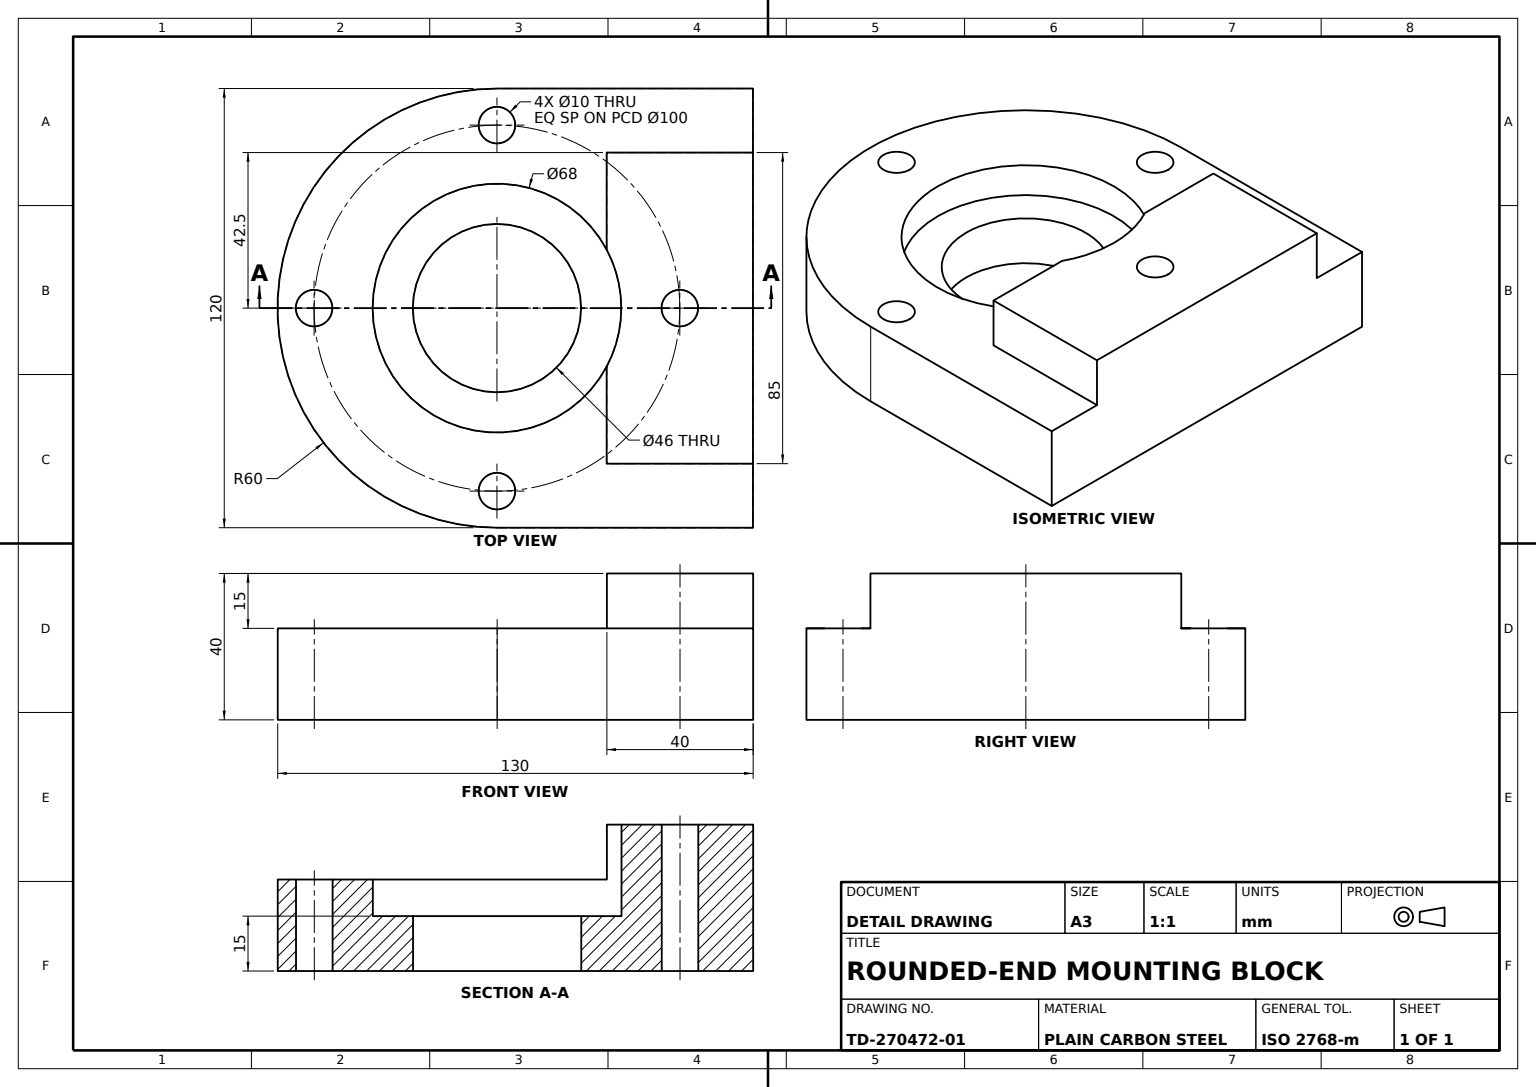
SolidWorks part; units mm, degrees
material "Plain Carbon Steel"
ref_plane "Front Plane" through (0, 0, 0) normal (0, 0, 1) x (1, 0, 0)
ref_plane "Top Plane" through (0, 0, 0) normal (0, 1, 0) x (1, 0, 0)
ref_plane "Right Plane" through (0, 0, 0) normal (1, 0, 0) x (0, 0, -1)
sketch "Base Plate Sketch" plane through (0, 0, 0) normal (0, 1, 0) x (1, 0, 0)
  line L0 (0, 35) -> (0, -35) construction
  line L1 (-60, 35) -> (60, 35)
  line L2 (-60, 35) -> (-60, -35)
  line L4 (60, 35) -> (60, -35)
  line L5 (-60, 35) -> (60, -35) construction
  line L6 (-60, -35) -> (60, 35) construction
  arc A1 (-60, -35) -> (60, -35) centre (0, -35) ccw
  point P0 (0, 0)
  dimension "D4" = 120
  dimension "D1" = 120
  dimension "D2" = 70
extrude "Base Plate" add sketch "Base Plate Sketch" along normal blind 25
sketch "Upright Block Sketch" plane through (0, 0, -35) normal (0, 0, -1) x (-1, 0, 0)
  line L0 (0, 0) -> (0, 48.3068) construction
  line L1 (-60, 25) -> (60, 25) construction
  line L2 (-42.5, 25) -> (42.5, 25)
  line L3 (-42.5, 25) -> (-42.5, 40)
  line L4 (-42.5, 40) -> (42.5, 40)
  line L5 (42.5, 25) -> (42.5, 40)
  dimension "D1" = 42.5
  dimension "D2" = 85
  dimension "D3" = 15
extrude "Upright Block" add sketch "Upright Block Sketch" against normal blind 40
sketch "Mounting Holes Sketch" plane through (0, 40, 0) normal (0, 1, 0) x (1, 0, 0)
  line L0 (0, 35) -> (0, -95) construction
  line L1 (-42.5, 35) -> (42.5, 35) construction
  line L2 (-26.3998, 15) -> (21.185, 15) construction
  line L3 (-60, -35) -> (60, -35) construction
  arc A0 (-60, -35) -> (60, -35) centre (0, -35) ccw construction
  circle A1 centre (0, 15) radius 5
  circle A2 centre (0, -35) radius 50 construction
  circle A3 centre (-50, -35) radius 5
  circle A4 centre (50, -35) radius 5
  circle A5 centre (0, -85) radius 5
  dimension "D2" = 10
  dimension "D4" = 100
  dimension "D5" = 10
  dimension "D1" = 20
  dimension "D3" = 20
extrude "Mounting Holes Cut" cut sketch "Mounting Holes Sketch" against normal blind 40
sketch "Counterbore Ø68 Sketch" plane through (0, 25, 0) normal (0, 1, 0) x (1, 0, 0)
  line L0 (0, 42.6024) -> (0, -115.8631) construction
  line L1 (-50, -35) -> (50, -35) construction
  circle A0 centre (0, -35) radius 34
  dimension "D1" = 68
extrude "Counterbore Ø68" cut sketch "Counterbore Ø68 Sketch" against normal blind 10 and the other way blind 40
sketch "Bore Ø46 Sketch" plane through (0, 15, 0) normal (0, 1, 0) x (1, 0, 0)
  line L0 (0, 40.1713) -> (0, -104.8678) construction
  line L1 (-50, -35) -> (50, -35) construction
  circle A0 centre (0, -35) radius 23
  dimension "D1" = 46
extrude "Bore Ø46" cut sketch "Bore Ø46 Sketch" against normal blind 15
